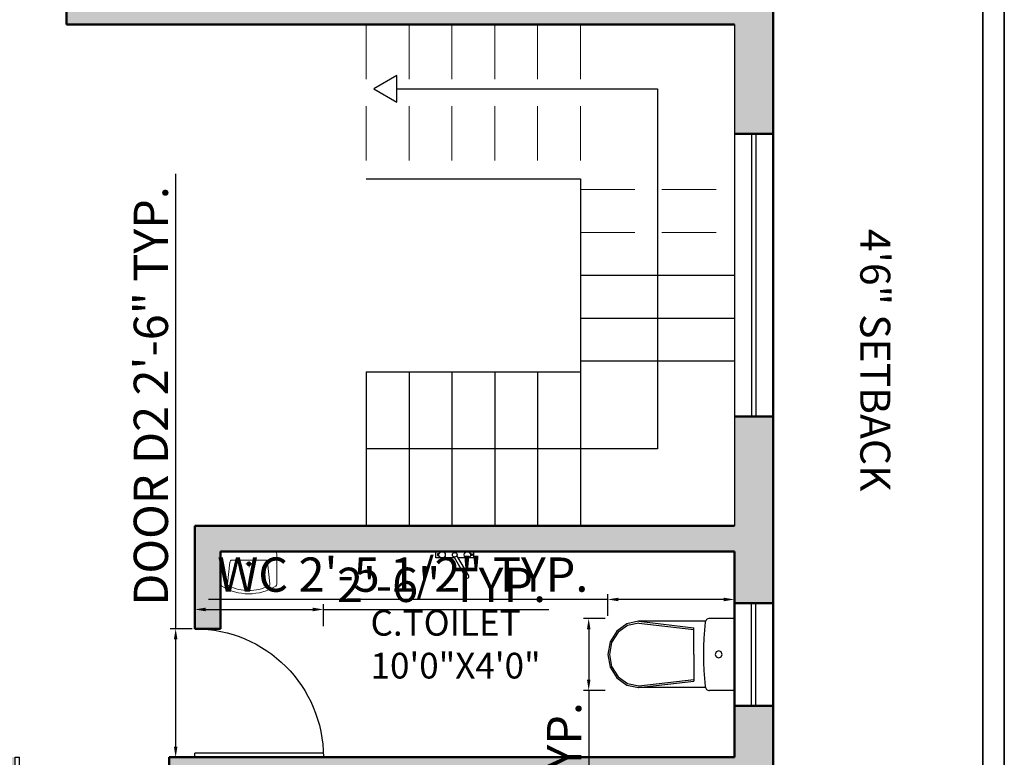
# Model space of a CAD drawing. Units: inches. Extents: x 3008 to 4088, y 1255 to 2137.
# Tile 28 of 30: x 3853 to 4083, y 1620 to 1792. Entities that reach past the tile are written whole.
import ezdxf

# ---------------------------------------------------------------- set-up
doc = ezdxf.new("R2010")
doc.units = ezdxf.units.IN
doc.linetypes.add('DASHED', pattern=[19.05, 12.7, -6.35])
for name, color, linetype, lineweight in [('A-ANNO-DIMS', 2, 'Continuous', 18), ('A-ANNO-TEXT', 7, 'Continuous', 18), ('A-AREA-IDEN', 7, 'Continuous', 18), ('A-DOOR', 4, 'Continuous', 25), ('A-FLOR-FIXT', 8, 'Continuous', 18), ('A-FLOR-STRS', 3, 'Continuous', 25), ('A-FLOR-STRS-OVHD', 3, 'DASHED', 18), ('A-GLAZ', 4, 'Continuous', 25), ('A-WALL', 7, 'Continuous', 50), ('A-WALL-PATT', 8, 'Continuous', 13), ('C-PROP', 1, 'Continuous', 35)]:
    doc.layers.add(name, color=color, linetype=linetype, lineweight=lineweight)
doc.layers.add('SANTEH', color=7, linetype='Continuous')
doc.styles.get("Standard").update_dxf_attribs({"font": 'arial.ttf'})
doc.dimstyles.new('ISO-25', dxfattribs={"dimtxt": 8, "dimasz": 2.5, "dimexe": 1.25, "dimexo": 0.625, "dimtad": 1, "dimdec": 1, "dimlunit": 3, "dimtxsty": 'Standard', "dimcen": 2.5, "dimadec": 0, "dimazin": 0, "dimtfac": 1, "dimtdec": 1, "dimtmove": 0, "dimatfit": 3, "dimfxl": 1, "dimarcsym": 0})

# ---------------------------------------------------------------- blocks, each defined once
blk = doc.blocks.new('D2')
for p, q in [((1722.5, 1505.46), (1722.5, 1475.46)), ((1723.5, 1505.46), (1723.5, 1475.46)), ((1722.5, 1475.46), (1723.5, 1475.46))]:
    blk.add_line(p, q)
blk.add_arc((1722.5, 1475.46), 30, 0, 90)
blk = doc.blocks.new('D1')
for p, q in [((1805.96, 1500.36), (1805.96, 1464.36)), ((1806.96, 1500.36), (1806.96, 1464.36)), ((1805.96, 1464.36), (1806.96, 1464.36))]:
    blk.add_line(p, q)
blk.add_arc((1805.96, 1464.36), 36, 0, 90)
blk = doc.blocks.new('WC 2 Symb_109')
at = {"layer": 'SANTEH'}
for p, q in [((0, 0), (0, 380)), ((0, 380), (132.4, 380)), ((153.6, 364.9), (506.8, 364.9)), ((506.3, 364.9), (215.7, 330.9)), ((506.3, 356), (215.7, 322)), ((215.7, 190), (215.7, 330.9)), ((215.7, 190), (215.7, 49.1)), ((506.3, 24), (215.7, 58)), ((153.8, 15.1), (506.8, 15.1)), ((506.3, 15.1), (215.7, 49.1)), ((0, 0), (132.4, 0))]:
    blk.add_line(p, q, dxfattribs=at)
for points in [[(154.6, 360.1), (153.9, 364.1), (152.3, 367.9), (150.2, 371.3), (147.4, 374.3), (144.1, 376.7), (140.5, 378.5), (136.5, 379.6), (132.4, 380)], [(506.8, 15.1), (569.2, 28.4), (622.2, 66.3), (657.6, 123.1), (670, 190), (657.6, 256.9), (622.2, 313.7), (569.2, 351.6), (506.8, 364.9)], [(154.6, 19.7), (158.6, 62.1), (161.4, 104.7), (163.1, 147.3), (163.7, 189.9), (163.1, 232.5), (161.4, 275.1), (158.6, 317.7), (154.6, 360.1)], [(506.3, 24), (565.5, 36.6), (615.7, 72.6), (649.2, 126.5), (661, 190), (649.2, 253.5), (615.7, 307.4), (565.5, 343.4), (506.3, 356)], [(132.4, 0), (136.5, 0.4), (140.4, 1.5), (144.1, 3.2), (147.3, 5.6), (150.1, 8.6), (152.3, 12), (153.8, 15.7), (154.6, 19.7)]]:
    blk.add_lwpolyline(points, dxfattribs=at)
blk.add_lwpolyline([(83.6, 208.5), (70.4, 203.1), (64.9, 190), (70.4, 176.9), (83.6, 171.5), (96.8, 176.9), (102.2, 190), (96.8, 203.1)], close=True, dxfattribs=at)
blk = doc.blocks.new('Faucet - kit sink top')
at = {"layer": 'SANTEH'}
for p, q in [((-5.5, -0.75), (-5.5, -1.25)), ((-4.94278, -0.75), (-5.5, -0.75)), ((-5.5, -1.25), (-4.94278, -1.25)), ((-0.14775, -1.7441), (3.56698, -8.1782)), ((4.43301, -7.6782), (0.71828, -1.2441)), ((4.94278, -0.75), (5.5, -0.75)), ((5.5, -1.25), (4.94278, -1.25)), ((5.5, -0.75), (5.5, -1.25))]:
    blk.add_line(p, q, dxfattribs=at)
blk.add_lwpolyline([(-0.00587, -2), (-6, -2), (-6, 0), (6, 0), (6, -2), (1.15195, -2)], dxfattribs=at)
for centre, radius in [((-4, -1), 1), ((4, -1), 1), ((0, -1), 0.75)]:
    blk.add_circle(centre, radius, dxfattribs=at)
blk.add_arc((4, -7.9282), 0.5, 210, 30, dxfattribs=at)
blk = doc.blocks.new('A$C2EBB240D')
for p, q in [((0, 355.8), (0, 86.6)), ((480, 375.8), (20, 375.8)), ((500, 355.8), (500, 86.6)), ((60.8, 89.8), (82.3, 282.2)), ((250, 300), (102.1, 300)), ((250, 300), (397.9, 300)), ((439.2, 89.8), (417.7, 282.2))]:
    blk.add_line(p, q)
for points in [[(275.2, 266.4), (219.4, 266.4)], [(247.3, 238.5), (247.3, 288.9)]]:
    blk.add_lwpolyline(points)
for centre, radius, start, end in [((20, 355.8), 20, 90, 180), ((480, 355.8), 20, 0, 90), ((102.1, 280), 20, 90, 173.64284), ((247.3, 266.4), 16.7, 90, 270), ((247.3, 266.4), 10, 90, 270), ((247.3, 266.4), 16.7, 270, 90), ((247.3, 266.4), 10, 270, 90), ((397.9, 280), 20, 6.35716, 90), ((80.7, 87.6), 20, 173.64284, 244.97956), ((419.3, 87.6), 20, 295.02044, 6.35716), ((20, 86.6), 20, 180, 237.68921), ((250, 450.3), 450.3, 237.68921, 270), ((250, 450.3), 420.3, 244.97956, 270), ((250, 450.3), 450.3, 270, 302.31079), ((250, 450.3), 420.3, 270, 295.02044), ((480, 86.6), 20, 302.31079, 0)]:
    blk.add_arc(centre, radius, start, end)
blk = doc.blocks.new('*D41')
at = {"layer": 'A-ANNO-DIMS', "color": 0, "lineweight": -2, "transparency": 16777216}
for p, q in [((3889.44, 1649.72), (3889.44, 1755.86)), ((3893.32, 1649.72), (3888.19, 1649.72)), ((3889.44, 1622.22), (3889.44, 1647.22)), ((3893.32, 1619.72), (3888.19, 1619.72))]:
    blk.add_line(p, q, dxfattribs=at)
at = {"layer": 'A-ANNO-DIMS', "color": 0, "transparency": 16777216}
for points in [[(3889.02, 1647.22), (3889.86, 1647.22), (3889.44, 1649.72)], [(3889.02, 1622.22), (3889.86, 1622.22), (3889.44, 1619.72)]]:
    blk.add_solid(points, dxfattribs=at)
at = {"layer": 'Defpoints', "color": 0, "transparency": 16777216}
for p in [(3889.44, 1649.72), (3893.94, 1649.72), (3893.94, 1619.72)]:
    blk.add_point(p, dxfattribs=at)
at = {"layer": 'A-ANNO-DIMS', "color": 0, "transparency": 16777216, "insert": (3884.68, 1704.04), "char_height": 8, "attachment_point": 5, "rotation": 90}
blk.add_mtext('DOOR D2 2\'-6" TYP.', dxfattribs=at)
blk = doc.blocks.new('*D42')
at = {"layer": 'A-ANNO-DIMS', "color": 0, "lineweight": -2, "transparency": 16777216}
for p, q in [((3893.94, 1650.35), (3893.94, 1655.47)), ((3923.94, 1650.35), (3923.94, 1655.47)), ((3896.44, 1654.22), (3921.44, 1654.22)), ((3923.94, 1654.22), (3976.59, 1654.22))]:
    blk.add_line(p, q, dxfattribs=at)
at = {"layer": 'A-ANNO-DIMS', "color": 0, "transparency": 16777216}
for points in [[(3896.44, 1654.64), (3896.44, 1653.8), (3893.94, 1654.22)], [(3921.44, 1654.64), (3921.44, 1653.8), (3923.94, 1654.22)]]:
    blk.add_solid(points, dxfattribs=at)
at = {"layer": 'Defpoints', "color": 0, "transparency": 16777216}
for p in [(3923.94, 1654.22), (3893.94, 1649.72), (3923.94, 1649.72)]:
    blk.add_point(p, dxfattribs=at)
at = {"layer": 'A-ANNO-DIMS', "color": 0, "transparency": 16777216, "insert": (3951.52, 1658.93), "char_height": 8, "attachment_point": 5}
blk.add_mtext('2\'-6" TYP.', dxfattribs=at)
blk = doc.blocks.new('*D45')
at = {"layer": 'A-ANNO-DIMS', "color": 0, "lineweight": -2, "transparency": 16777216}
for p, q in [((3990.33, 1652.74), (3990.33, 1657.81)), ((4019.94, 1652.74), (4019.94, 1657.81)), ((3990.33, 1656.56), (3897.13, 1656.56)), ((4017.44, 1656.56), (3992.83, 1656.56))]:
    blk.add_line(p, q, dxfattribs=at)
at = {"layer": 'A-ANNO-DIMS', "color": 0, "transparency": 16777216}
for points in [[(3992.83, 1656.97), (3992.83, 1656.14), (3990.33, 1656.56)], [(4017.44, 1656.97), (4017.44, 1656.14), (4019.94, 1656.56)]]:
    blk.add_solid(points, dxfattribs=at)
at = {"layer": 'Defpoints', "color": 0, "transparency": 16777216}
for p in [(3990.33, 1656.56), (3990.33, 1652.12), (4019.94, 1652.12)]:
    blk.add_point(p, dxfattribs=at)
at = {"layer": 'A-ANNO-DIMS', "color": 0, "transparency": 16777216, "insert": (3942.48, 1661.32), "char_height": 8, "attachment_point": 5}
blk.add_mtext('WC 2\'-5 1/2" TYP.', dxfattribs=at)
blk = doc.blocks.new('*D46')
at = {"layer": 'A-ANNO-DIMS', "color": 0, "lineweight": -2, "transparency": 16777216}
for p, q in [((3989.71, 1652.12), (3984.64, 1652.12)), ((3985.89, 1649.62), (3985.89, 1637.82)), ((3989.71, 1635.32), (3984.64, 1635.32)), ((3985.89, 1635.32), (3985.89, 1583.56))]:
    blk.add_line(p, q, dxfattribs=at)
at = {"layer": 'A-ANNO-DIMS', "color": 0, "transparency": 16777216}
for points in [[(3985.48, 1649.62), (3986.31, 1649.62), (3985.89, 1652.12)], [(3985.48, 1637.82), (3986.31, 1637.82), (3985.89, 1635.32)]]:
    blk.add_solid(points, dxfattribs=at)
at = {"layer": 'Defpoints', "color": 0, "transparency": 16777216}
for p in [(3990.33, 1652.12), (3985.89, 1635.32), (3990.33, 1635.32)]:
    blk.add_point(p, dxfattribs=at)
at = {"layer": 'A-ANNO-DIMS', "color": 0, "transparency": 16777216, "insert": (3981.18, 1608.19), "char_height": 8, "attachment_point": 5, "rotation": 90}
blk.add_mtext('1\'-5" TYP.', dxfattribs=at)

msp = doc.modelspace()

# ---------------------------------------------------------------- hatches: boundary and pattern name
at = {"layer": 'A-WALL-PATT'}
h = msp.add_hatch(color=256, dxfattribs=at)
h.dxf.hatch_style = 1
h.paths.add_polyline_path([(3665.94, 1631.72), (3656.94, 1631.72), (3656.94, 1546.72), (3665.94, 1546.72)])
h.paths.add_polyline_path([(3851.94, 1619.72), (3701.94, 1619.72), (3701.94, 1610.72), (3788.94, 1610.72), (3788.94, 1469.72), (3809.94, 1469.72), (3809.94, 1478.72), (3797.94, 1478.72), (3797.94, 1550.72), (3815.94, 1550.72), (3815.94, 1556.72), (3797.94, 1556.72), (3797.94, 1610.72), (3845.94, 1610.72), (3845.94, 1586.72), (3851.94, 1586.72)])
h.paths.add_polyline_path([(4028.94, 1631.72), (4019.94, 1631.72), (4019.94, 1619.72), (3887.94, 1619.72), (3887.94, 1610.72), (4019.94, 1610.72), (4019.94, 1577.72), (4028.94, 1577.72)])
h.paths.add_polyline_path([(3875.94, 1478.72), (3851.94, 1478.72), (3851.94, 1556.72), (3845.94, 1556.72), (3845.94, 1526.72), (3845.94, 1478.72), (3833.94, 1478.72), (3833.94, 1469.72), (3875.94, 1469.72)])
h.paths.add_polyline_path([(3959.94, 1478.72), (3917.94, 1478.72), (3917.94, 1469.72), (3959.94, 1469.72)])
h.paths.add_polyline_path([(4028.94, 1511.72), (4019.94, 1511.72), (4019.94, 1478.72), (4001.94, 1478.72), (4001.94, 1469.72), (4028.94, 1469.72)])
h.paths.add_polyline_path([(4028.94, 1699.22), (4019.94, 1699.22), (4019.94, 1673.72), (3893.94, 1673.72), (3893.94, 1649.72), (3899.94, 1649.72), (3899.94, 1667.72), (4019.94, 1667.72), (4019.94, 1655.72), (4028.94, 1655.72)])
h.paths.add_polyline_path([(4028.94, 1847.72), (4019.94, 1847.72), (4019.94, 1796.72), (3863.94, 1796.72), (3863.94, 1790.72), (4019.94, 1790.72), (4019.94, 1765.22), (4028.94, 1765.22)])
h.paths.add_polyline_path([(3815.94, 1796.72), (3779.94, 1796.72), (3665.94, 1796.72), (3665.94, 1898.72), (3656.94, 1898.72), (3656.94, 1673.72), (3665.94, 1673.72), (3665.94, 1790.72), (3815.94, 1790.72)])
h.paths.add_polyline_path([(3755.94, 1949.72), (3656.94, 1949.72), (3656.94, 1940.72), (3665.94, 1940.72), (3755.94, 1940.72)])
h.paths.add_polyline_path([(3827.94, 1949.72), (3797.94, 1949.72), (3797.94, 1940.72), (3809.94, 1940.72), (3809.94, 1874.72), (3815.94, 1874.72), (3815.94, 1940.72), (3827.94, 1940.72)])
h.paths.add_polyline_path([(3953.94, 1949.72), (3851.94, 1949.72), (3851.94, 1940.72), (3863.94, 1940.72), (3863.94, 1844.72), (3809.94, 1844.72), (3809.94, 1832.72), (3815.94, 1832.72), (3815.94, 1838.72), (3863.94, 1838.72), (3869.94, 1838.72), (3869.94, 1940.72), (3953.94, 1940.72)])
h.paths.add_polyline_path([(4028.94, 1949.72), (3995.94, 1949.72), (3995.94, 1940.72), (4019.94, 1940.72), (4019.94, 1889.72), (4028.94, 1889.72)])

# ---------------------------------------------------------------- linework, layer by layer
at = {"layer": 'A-FLOR-STRS'}
for p, q in [((4019.94, 1790.72), (4019.94, 1673.72)), ((3933.94, 1754.72), (3983.94, 1754.72)), ((3983.94, 1754.72), (3983.94, 1673.72)), ((3983.94, 1732.22), (4019.94, 1732.22)), ((3983.94, 1722.22), (4019.94, 1722.22)), ((3983.94, 1712.22), (4019.94, 1712.22)), ((3933.94, 1709.72), (3983.94, 1709.72)), ((3933.94, 1709.72), (3933.94, 1673.72)), ((3943.94, 1709.72), (3943.94, 1673.72)), ((3953.94, 1709.72), (3953.94, 1673.72)), ((3963.94, 1709.72), (3963.94, 1673.72)), ((3973.94, 1709.72), (3973.94, 1673.72))]:
    msp.add_line(p, q, dxfattribs=at)
msp.add_lwpolyline([(3935.73, 1775.72), (3941.08, 1772.63), (3941.08, 1778.81)], close=True, dxfattribs=at)
msp.add_lwpolyline([(3941.08, 1775.72), (4001.94, 1775.72), (4001.94, 1691.72), (3933.94, 1691.72)], dxfattribs=at)
at = {"layer": 'A-FLOR-STRS-OVHD'}
for p, q in [((3933.94, 1790.72), (3933.94, 1754.72)), ((3943.94, 1790.72), (3943.94, 1754.72)), ((3953.94, 1790.72), (3953.94, 1754.72)), ((3963.94, 1790.72), (3963.94, 1754.72)), ((3973.94, 1790.72), (3973.94, 1754.72)), ((3983.94, 1790.72), (3983.94, 1754.72)), ((3983.94, 1752.22), (4019.94, 1752.22)), ((3983.94, 1742.22), (4019.94, 1742.22))]:
    msp.add_line(p, q, dxfattribs=at)
at = {"layer": 'A-GLAZ'}
for p, q in [((4023.94, 1765.22), (4023.94, 1699.22)), ((4023.94, 1765.22), (4023.94, 1699.22)), ((4024.94, 1765.22), (4024.94, 1699.22)), ((4023.94, 1631.72), (4023.94, 1655.72)), ((4024.94, 1631.72), (4024.94, 1655.72))]:
    msp.add_line(p, q, dxfattribs=at)
at = {"layer": 'A-WALL'}
for p, q in [((4028.94, 1949.72), (4028.94, 1469.72)), ((3863.94, 1796.72), (3863.94, 1790.72)), ((3863.94, 1790.72), (4019.94, 1790.72)), ((4019.94, 1765.22), (4028.94, 1765.22)), ((4019.94, 1699.22), (4028.94, 1699.22)), ((3893.94, 1673.72), (4019.94, 1673.72)), ((3893.94, 1673.72), (3893.94, 1649.72)), ((3899.94, 1667.72), (4019.94, 1667.72)), ((3899.94, 1667.72), (3899.94, 1649.72)), ((4019.94, 1667.72), (4019.94, 1619.72)), ((4019.94, 1655.72), (4028.94, 1655.72)), ((3893.94, 1649.72), (3899.94, 1649.72)), ((4019.94, 1631.72), (4028.94, 1631.72)), ((3887.94, 1619.72), (4019.94, 1619.72)), ((3887.94, 1610.72), (3887.94, 1619.72))]:
    msp.add_line(p, q, dxfattribs=at)
at = {"layer": 'C-PROP'}
for p, q in [((4082.94, 2009.72), (4082.94, 1349.72)), ((4077.94, 2004.72), (4077.94, 1354.72))]:
    msp.add_line(p, q, dxfattribs=at)

# ---------------------------------------------------------------- block references
at = {"layer": 'A-DOOR', "xscale": -1}
for name, p, rotation in [('D2', (2418.48, -102.78), 270), ('D1', (2045.98, 3084.08), 180)]:
    msp.add_blockref(name, p, dxfattribs=dict(at, rotation=rotation))
at = {"layer": 'A-FLOR-FIXT'}
for name, p, xscale, yscale, zscale in [('A$C2EBB240D', (3913.05, 1657.87), -0.026211548048557, 0.026211548048557, 0.026211548048557), ('Faucet - kit sink top', (3954.6, 1667.72), 0.7356136897818673, 0.7356136897818673, 0.7356136897818673)]:
    msp.add_blockref(name, p, dxfattribs=dict(at, xscale=xscale, yscale=yscale, zscale=zscale))
at = {"layer": 'A-FLOR-FIXT', "xscale": 0.0441898926459964, "yscale": 0.0441898926459964, "zscale": 0.0441898926459964, "rotation": 180}
msp.add_blockref('WC 2 Symb_109', (4019.94, 1652.12), dxfattribs=at)

# ---------------------------------------------------------------- texts
at = {"layer": 'A-ANNO-TEXT', "insert": (4056.31, 1743.06), "char_height": 7, "attachment_point": 1, "rotation": 270}
msp.add_mtext_dynamic_manual_height_columns('{\\fTimes New Roman|b0|i0|c0|p18;4\'6" SETBACK}', width=105.6127, gutter_width=12.5, heights=[0], dxfattribs=at)
at = {"layer": 'A-AREA-IDEN', "insert": (3934.95, 1654.11), "char_height": 6, "attachment_point": 1}
msp.add_mtext_dynamic_manual_height_columns('{\\fTimes New Roman|b0|i0|c0|p18;C.TOILET\\P10\'0"X4\'0"}', width=105.6127, gutter_width=12.5, heights=[0], dxfattribs=at)

# ---------------------------------------------------------------- dimensions: what is measured, and where the dimension line sits
at = {"layer": 'A-ANNO-DIMS'}
for base, p1, p2, angle, text, picture, middle in [((3889.44, 1649.72), (3893.94, 1619.72), (3893.94, 1649.72), 90, 'DOOR D2 <> TYP.', '*D41', (3884.68, 1704.04)), ((3990.33, 1656.56), (4019.94, 1652.12), (3990.33, 1652.12), 180, 'WC <> TYP.', '*D45', (3942.48, 1661.32)), ((3985.89, 1635.32), (3990.33, 1652.12), (3990.33, 1635.32), 270, '<> TYP.', '*D46', (3981.18, 1608.19))]:
    dim = msp.add_linear_dim(base=base, p1=p1, p2=p2, angle=angle, text=text, dimstyle='ISO-25', override={"dimdec": 1, "dimrnd": 0, "dimzin": 1, "dimlunit": 4, "dimfrac": 2}, dxfattribs=at)
    dim.commit()
    dim.dimension.update_dxf_attribs({"geometry": picture, "text_midpoint": middle})
dim = msp.add_linear_dim(base=(3923.94, 1654.22), p1=(3893.94, 1649.72), p2=(3923.94, 1649.72), text='<> TYP.', dimstyle='ISO-25', override={"dimdec": 1, "dimrnd": 0, "dimzin": 1, "dimlunit": 4, "dimfrac": 2}, dxfattribs=at)
dim.commit()
dim.dimension.update_dxf_attribs({"geometry": '*D42', "text_midpoint": (3951.52, 1658.93)})

doc.saveas('drawing.dxf')
